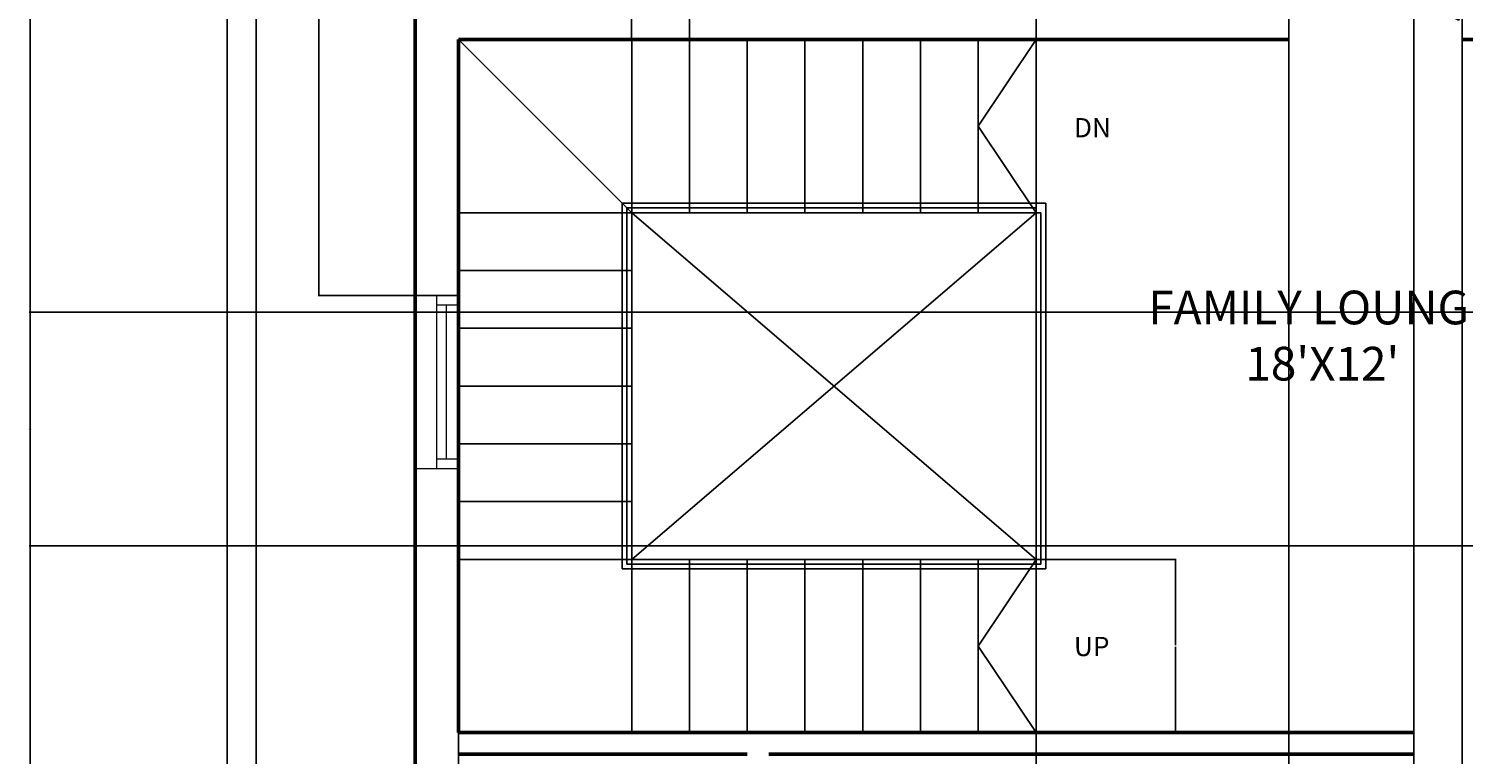
# Model space of a CAD drawing. Units: inches. Extents: x -28 to 483, y -584 to 51.
# Tile 2 of 6: x -28 to 270, y -342 to -191. Entities that reach past the tile are written whole.
import ezdxf

# ---------------------------------------------------------------- set-up
doc = ezdxf.new("R2010")
doc.units = ezdxf.units.IN
doc.header["$MEASUREMENT"] = 0
for name, color, linetype, lineweight in [('A-ANNO-DIMS', 2, 'Continuous', 18), ('A-ANNO-TEXT', 7, 'Continuous', 18), ('A-AREA-IDEN', 7, 'Continuous', 25), ('A-DOOR', 4, 'Continuous', 25), ('A-FLOR-STRS', 7, 'Continuous', 25), ('A-GLAZ', 5, 'Continuous', 18), ('A-WALL', 7, 'Continuous', 50), ('C-PROP', 7, 'Continuous', 25)]:
    doc.layers.add(name, color=color, linetype=linetype, lineweight=lineweight)
doc.styles.get("Standard").update_dxf_attribs({"font": 'arial.ttf'})
doc.dimstyles.get("Standard").update_dxf_attribs({"dimtxt": 0.18, "dimasz": 0.18, "dimexe": 0.18, "dimexo": 0.0625, "dimgap": 0.09, "dimtad": 0, "dimtih": 1, "dimtoh": 1, "dimdec": 4, "dimzin": 0, "dimdsep": 46, "dimtxsty": 'Standard', "dimcen": 0.09, "dimadec": 0, "dimazin": 0, "dimtfac": 1, "dimtdec": 4, "dimtofl": 0, "dimtmove": 0, "dimatfit": 3, "dimfxl": 1, "dimtolj": 1, "dimtzin": 0, "dimarcsym": 0})

# ---------------------------------------------------------------- blocks, each defined once
blk = doc.blocks.new('*U2')
for p, q in [((0, 0), (0, -6)), ((40, 0), (40, -6))]:
    blk.add_line(p, q)
blk.add_lwpolyline([(0, 0), (34.64, 20), (35.52, 18.48), (0.87, -1.52)], close=True)
blk.add_arc((0, 0), 40, 0, 30)
blk = doc.blocks.new('WIN-36IN')
for p, q in [((0, 9), (0, 0)), ((2, 9), (2, 4.5)), ((34, 9), (34, 4.5)), ((36, 9), (36, 0)), ((34, 6.5), (2, 6.5)), ((36, 4.5), (0, 4.5))]:
    blk.add_line(p, q)
blk = doc.blocks.new('*D20')
at = {"layer": 'A-ANNO-DIMS', "color": 0, "lineweight": -2, "transparency": 16777216}
for p, q in [((12.78, 21.41), (-28.29, 21.41)), ((-28.11, 21.23), (-28.11, -266.41)), ((-28.11, -554.41), (-28.11, -266.77)), ((12.78, -554.59), (-28.29, -554.59))]:
    blk.add_line(p, q, dxfattribs=at)
at = {"layer": 'A-ANNO-DIMS', "color": 0, "transparency": 16777216}
for points in [[(-28.14, 21.23), (-28.08, 21.23), (-28.11, 21.41)], [(-28.14, -554.41), (-28.08, -554.41), (-28.11, -554.59)]]:
    blk.add_solid(points, dxfattribs=at)
at = {"layer": 'Defpoints', "color": 0, "transparency": 16777216}
for p in [(-28.11, 21.41), (12.84, 21.41), (12.84, -554.59)]:
    blk.add_point(p, dxfattribs=at)
at = {"layer": 'A-ANNO-DIMS', "color": 0, "transparency": 16777216, "insert": (-28.11, -266.59), "char_height": 0.18, "attachment_point": 5}
blk.add_mtext('\\A1;576', dxfattribs=at)
blk = doc.blocks.new('*D26')
at = {"layer": 'A-ANNO-DIMS', "color": 0, "lineweight": -2, "transparency": 16777216}
for p, q in [((60.84, -337.15), (60.84, -583.72)), ((180.84, -337.15), (180.84, -583.72)), ((61.02, -583.54), (120.56, -583.54)), ((180.66, -583.54), (121.12, -583.54))]:
    blk.add_line(p, q, dxfattribs=at)
at = {"layer": 'A-ANNO-DIMS', "color": 0, "transparency": 16777216}
for points in [[(61.02, -583.51), (61.02, -583.57), (60.84, -583.54)], [(180.66, -583.51), (180.66, -583.57), (180.84, -583.54)]]:
    blk.add_solid(points, dxfattribs=at)
at = {"layer": 'Defpoints', "color": 0, "transparency": 16777216}
for p in [(60.84, -337.09), (180.84, -337.09), (180.84, -583.54)]:
    blk.add_point(p, dxfattribs=at)
at = {"layer": 'A-ANNO-DIMS', "color": 0, "transparency": 16777216, "insert": (120.84, -583.54), "char_height": 0.18, "attachment_point": 5}
blk.add_mtext('\\A1;120', dxfattribs=at)
blk = doc.blocks.new('*D27')
at = {"layer": 'A-ANNO-DIMS', "color": 0, "lineweight": -2, "transparency": 16777216}
for p, q in [((180.91, -301.09), (209.97, -301.09)), ((209.79, -301.27), (209.79, -318.91)), ((209.79, -336.91), (209.79, -319.27)), ((180.91, -337.09), (209.97, -337.09))]:
    blk.add_line(p, q, dxfattribs=at)
at = {"layer": 'A-ANNO-DIMS', "color": 0, "transparency": 16777216}
for points in [[(209.76, -301.27), (209.82, -301.27), (209.79, -301.09)], [(209.76, -336.91), (209.82, -336.91), (209.79, -337.09)]]:
    blk.add_solid(points, dxfattribs=at)
at = {"layer": 'Defpoints', "color": 0, "transparency": 16777216}
for p in [(180.84, -301.09), (180.84, -337.09), (209.79, -337.09)]:
    blk.add_point(p, dxfattribs=at)
at = {"layer": 'A-ANNO-DIMS', "color": 0, "transparency": 16777216, "insert": (209.79, -319.09), "char_height": 0.18, "attachment_point": 5}
blk.add_mtext('\\A1;36', dxfattribs=at)
blk = doc.blocks.new('*D28')
at = {"layer": 'A-ANNO-DIMS', "color": 0, "lineweight": -2, "transparency": 16777216}
for p, q in [((233.35, -193.15), (233.35, -583.72)), ((269.35, -193.15), (269.35, -583.72)), ((233.53, -583.54), (251.13, -583.54)), ((269.17, -583.54), (251.57, -583.54))]:
    blk.add_line(p, q, dxfattribs=at)
at = {"layer": 'A-ANNO-DIMS', "color": 0, "transparency": 16777216}
for points in [[(233.53, -583.51), (233.53, -583.57), (233.35, -583.54)], [(269.17, -583.51), (269.17, -583.57), (269.35, -583.54)]]:
    blk.add_solid(points, dxfattribs=at)
at = {"layer": 'Defpoints', "color": 0, "transparency": 16777216}
for p in [(233.35, -193.09), (269.35, -193.09), (269.35, -583.54)]:
    blk.add_point(p, dxfattribs=at)
at = {"layer": 'A-ANNO-DIMS', "color": 0, "transparency": 16777216, "insert": (251.35, -583.54), "char_height": 0.18, "attachment_point": 5}
blk.add_mtext('\\A1;36', dxfattribs=at)
blk = doc.blocks.new('*D34')
at = {"layer": 'A-ANNO-DIMS', "color": 0, "lineweight": -2, "transparency": 16777216}
for p, q in [((60.78, -130.91), (31.71, -130.91)), ((31.89, -131.09), (31.89, -188.42)), ((31.89, -246.11), (31.89, -188.78)), ((60.78, -246.29), (31.71, -246.29))]:
    blk.add_line(p, q, dxfattribs=at)
at = {"layer": 'A-ANNO-DIMS', "color": 0, "transparency": 16777216}
for points in [[(31.86, -131.09), (31.92, -131.09), (31.89, -130.91)], [(31.86, -246.11), (31.92, -246.11), (31.89, -246.29)]]:
    blk.add_solid(points, dxfattribs=at)
at = {"layer": 'Defpoints', "color": 0, "transparency": 16777216}
for p in [(31.89, -130.91), (60.84, -130.91), (60.84, -246.29)]:
    blk.add_point(p, dxfattribs=at)
at = {"layer": 'A-ANNO-DIMS', "color": 0, "transparency": 16777216, "insert": (31.89, -188.6), "char_height": 0.18, "attachment_point": 5}
blk.add_mtext('\\A1;115.39', dxfattribs=at)
blk = doc.blocks.new('*D38')
at = {"layer": 'A-ANNO-DIMS', "color": 0, "lineweight": -2, "transparency": 16777216}
for p, q in [((296.28, -249.73), (-28.29, -249.73)), ((-28.11, -249.91), (-28.11, -273.82)), ((-28.11, -298.1), (-28.11, -274.19)), ((296.28, -298.28), (-28.29, -298.28))]:
    blk.add_line(p, q, dxfattribs=at)
at = {"layer": 'A-ANNO-DIMS', "color": 0, "transparency": 16777216}
for points in [[(-28.14, -249.91), (-28.08, -249.91), (-28.11, -249.73)], [(-28.14, -298.1), (-28.08, -298.1), (-28.11, -298.28)]]:
    blk.add_solid(points, dxfattribs=at)
at = {"layer": 'Defpoints', "color": 0, "transparency": 16777216}
for p in [(296.34, -249.73), (-28.11, -298.28), (296.34, -298.28)]:
    blk.add_point(p, dxfattribs=at)
at = {"layer": 'A-ANNO-DIMS', "color": 0, "transparency": 16777216, "insert": (-28.11, -274), "char_height": 0.18, "attachment_point": 5}
blk.add_mtext('\\A1;48.54', dxfattribs=at)
blk = doc.blocks.new('*D46')
at = {"layer": 'A-ANNO-DIMS', "color": 0, "lineweight": -2, "transparency": 16777216}
for p, q in [((180.84, -337.03), (180.84, 50.54)), ((181.02, 50.36), (219.68, 50.36)), ((259.11, 50.36), (220.46, 50.36)), ((259.29, -337.03), (259.29, 50.54))]:
    blk.add_line(p, q, dxfattribs=at)
at = {"layer": 'A-ANNO-DIMS', "color": 0, "transparency": 16777216}
for points in [[(181.02, 50.39), (181.02, 50.33), (180.84, 50.36)], [(259.11, 50.39), (259.11, 50.33), (259.29, 50.36)]]:
    blk.add_solid(points, dxfattribs=at)
at = {"layer": 'Defpoints', "color": 0, "transparency": 16777216}
for p in [(259.29, 50.36), (180.84, -337.09), (259.29, -337.09)]:
    blk.add_point(p, dxfattribs=at)
at = {"layer": 'A-ANNO-DIMS', "color": 0, "transparency": 16777216, "insert": (220.07, 50.36), "char_height": 0.18, "attachment_point": 5}
blk.add_mtext('\\A1;78.45', dxfattribs=at)
blk = doc.blocks.new('*D48')
at = {"layer": 'A-ANNO-DIMS', "color": 0, "lineweight": -2, "transparency": 16777216}
for p, q in [((96.84, -193.03), (96.84, -163.96)), ((97.02, -164.14), (102.63, -164.14)), ((108.66, -164.14), (103.05, -164.14)), ((108.84, -193.03), (108.84, -163.96))]:
    blk.add_line(p, q, dxfattribs=at)
at = {"layer": 'A-ANNO-DIMS', "color": 0, "transparency": 16777216}
for points in [[(97.02, -164.11), (97.02, -164.17), (96.84, -164.14)], [(108.66, -164.11), (108.66, -164.17), (108.84, -164.14)]]:
    blk.add_solid(points, dxfattribs=at)
at = {"layer": 'Defpoints', "color": 0, "transparency": 16777216}
for p in [(108.84, -164.14), (96.84, -193.09), (108.84, -193.09)]:
    blk.add_point(p, dxfattribs=at)
at = {"layer": 'A-ANNO-DIMS', "color": 0, "transparency": 16777216, "insert": (102.84, -164.14), "char_height": 0.18, "attachment_point": 5}
blk.add_mtext('\\A1;12', dxfattribs=at)

msp = doc.modelspace()

# ---------------------------------------------------------------- linework, layer by layer
at = {"layer": 'A-FLOR-STRS'}
for p, q in [((96.8432, -229.0877), (60.8432, -193.0877)), ((96.8432, -193.0877), (96.8432, -229.0877)), ((108.8432, -193.0877), (108.8432, -229.0877)), ((120.8432, -193.0877), (120.8432, -229.0877)), ((132.8432, -193.0877), (132.8432, -229.0877)), ((144.8432, -193.0877), (144.8432, -229.0877)), ((156.8432, -193.0877), (156.8432, -229.0877)), ((168.8432, -193.0877), (168.8432, -229.0877)), ((180.8432, -193.0877), (168.8432, -211.0877)), ((180.8432, -193.0877), (180.8432, -229.0877)), ((168.8432, -211.0877), (180.8432, -229.0877)), ((96.8432, -229.0877), (60.8432, -229.0877)), ((94.8432, -303.0877), (94.8432, -227.0877)), ((94.8432, -227.0877), (182.8432, -227.0877)), ((95.8432, -302.0877), (95.8432, -228.0877)), ((95.8432, -228.0877), (180.8432, -228.0877)), ((96.8432, -301.0877), (96.8432, -229.0877)), ((96.8432, -229.0877), (181.8432, -229.0877)), ((96.8432, -229.0877), (180.8432, -301.0877)), ((96.8432, -301.0877), (180.8432, -229.0877)), ((180.8432, -229.0877), (180.8432, -301.0877)), ((181.8432, -229.0877), (181.8432, -302.0877)), ((182.8432, -227.0877), (182.8432, -303.0877)), ((96.8432, -241.0877), (60.8432, -241.0877)), ((96.8432, -253.0877), (60.8432, -253.0877)), ((96.8432, -265.0877), (60.8432, -265.0877)), ((96.8432, -277.0877), (60.8432, -277.0877)), ((96.8432, -289.0877), (60.8432, -289.0877)), ((96.8432, -301.0877), (60.8432, -301.0877)), ((182.8432, -303.0877), (94.8432, -303.0877)), ((181.8432, -302.0877), (95.8432, -302.0877)), ((96.8432, -337.0877), (96.8432, -301.0877)), ((180.8432, -301.0877), (96.8432, -301.0877)), ((108.8432, -337.0877), (108.8432, -301.0877)), ((120.8432, -337.0877), (120.8432, -301.0877)), ((132.8432, -337.0877), (132.8432, -301.0877)), ((144.8432, -337.0877), (144.8432, -301.0877)), ((156.8432, -337.0877), (156.8432, -301.0877)), ((168.8432, -337.0877), (168.8432, -301.0877)), ((180.8432, -301.0877), (168.8432, -319.0877)), ((180.8432, -337.0877), (180.8432, -301.0877)), ((168.8432, -319.0877), (180.8432, -337.0877))]:
    msp.add_line(p, q, dxfattribs=at)
at = {"layer": 'A-WALL'}
for p, q in [((51.8432, -17.5877), (51.8432, -494.5877)), ((60.8432, -193.0877), (233.3523, -193.0877)), ((60.8432, -193.0877), (60.8432, -337.0877)), ((269.3523, -193.0877), (393.8432, -193.0877)), ((60.8432, -337.0877), (259.2944, -337.0877)), ((60.8432, -341.5877), (120.8432, -341.5877)), ((125.3432, -341.5877), (259.2944, -341.5877))]:
    msp.add_line(p, q, dxfattribs=at)
at = {"layer": 'C-PROP'}
for p, q in [((12.8432, 21.4123), (12.8432, -554.5877)), ((18.8432, 15.4123), (18.8432, -548.5877))]:
    msp.add_line(p, q, dxfattribs=at)

# ---------------------------------------------------------------- block references
at = {"layer": 'A-DOOR', "xscale": -0.9, "yscale": 0.9, "zscale": 0.9}
msp.add_blockref('*U2', (269.3523, -187.6877), dxfattribs=at)
at = {"layer": 'A-DOOR', "xscale": 0.9, "yscale": 0.9, "zscale": 0.9, "rotation": 180}
msp.add_blockref('*U2', (295.2944, -342.4877), dxfattribs=at)
at = {"layer": 'A-GLAZ', "rotation": 269.9999999999998}
msp.add_blockref('WIN-36IN', (51.8428, -246.2923), dxfattribs=at)

# ---------------------------------------------------------------- texts
at = {"layer": 'A-ANNO-TEXT', "char_height": 4, "attachment_point": 1}
for s, insert in [('DN', (188.7109, -209.4094)), ('UP', (188.7109, -317.1863))]:
    msp.add_mtext_dynamic_manual_height_columns(s, width=23.645684, gutter_width=1, heights=[0], dxfattribs=dict(at, insert=insert))
at = {"layer": 'A-AREA-IDEN', "insert": (189.5927, -245.2647), "char_height": 7, "attachment_point": 1}
msp.add_mtext_dynamic_manual_height_columns("\\pxqc;FAMILY LOUNGE\\P18'X12'", width=101.426885, gutter_width=1, heights=[0], dxfattribs=at)

# ---------------------------------------------------------------- dimensions: what is measured, and where the dimension line sits
at = {"layer": 'A-ANNO-DIMS'}
for base, p1, p2, override, picture, middle in [((259.2944, 50.3623), (180.8432, -337.0877), (259.2944, -337.0877), {"dimdec": 2, "dimlfac": 1, "dimrnd": 0, "dimzin": 0, "dimdsep": 46, "dimlunit": 2}, '*D46', (220.0688, 50.3623)), ((108.8432, -164.1377), (96.8432, -193.0877), (108.8432, -193.0877), {"dimdec": 0, "dimlfac": 1, "dimrnd": 0, "dimzin": 0, "dimdsep": 46, "dimlunit": 2}, '*D48', (102.8432, -164.1377)), ((269.3523, -583.5377), (233.3523, -193.0877), (269.3523, -193.0877), {"dimdec": 0, "dimlfac": 1, "dimrnd": 0, "dimzin": 0, "dimdsep": 46, "dimlunit": 2}, '*D28', (251.3523, -583.5377)), ((180.8432, -583.5377), (60.8432, -337.0877), (180.8432, -337.0877), {"dimdec": 0, "dimlfac": 1, "dimrnd": 0, "dimzin": 0, "dimdsep": 46, "dimlunit": 2}, '*D26', (120.8432, -583.5377))]:
    dim = msp.add_linear_dim(base=base, p1=p1, p2=p2, dimstyle='Standard', override=override, dxfattribs=at)
    dim.commit()
    dim.dimension.update_dxf_attribs({"geometry": picture, "text_midpoint": middle})
for base, p1, p2, angle, override, picture, middle in [((-28.1068, 21.4123), (12.8432, -554.5877), (12.8432, 21.4123), 90, {"dimdec": 0, "dimlfac": 1, "dimrnd": 0, "dimzin": 0, "dimdsep": 46, "dimlunit": 2}, '*D20', (-28.1068, -266.5877)), ((31.8932, -130.9071), (60.8432, -246.2923), (60.8432, -130.9071), 90, {"dimdec": 2, "dimlfac": 1, "dimrnd": 0, "dimzin": 0, "dimdsep": 46, "dimlunit": 2}, '*D34', (31.8932, -188.5997)), ((-28.1068, -298.276), (296.3395, -249.7333), (296.3395, -298.276), 90, {"dimdec": 2, "dimlfac": 1, "dimrnd": 0, "dimzin": 0, "dimdsep": 46, "dimlunit": 2}, '*D38', (-28.1068, -274.0046)), ((209.7932, -337.0877), (180.8432, -301.0877), (180.8432, -337.0877), 270, {"dimdec": 0, "dimlfac": 1, "dimrnd": 0, "dimzin": 0, "dimdsep": 46, "dimlunit": 2}, '*D27', (209.7932, -319.0877))]:
    dim = msp.add_linear_dim(base=base, p1=p1, p2=p2, angle=angle, dimstyle='Standard', override=override, dxfattribs=at)
    dim.commit()
    dim.dimension.update_dxf_attribs({"geometry": picture, "text_midpoint": middle})

doc.saveas('drawing.dxf')
